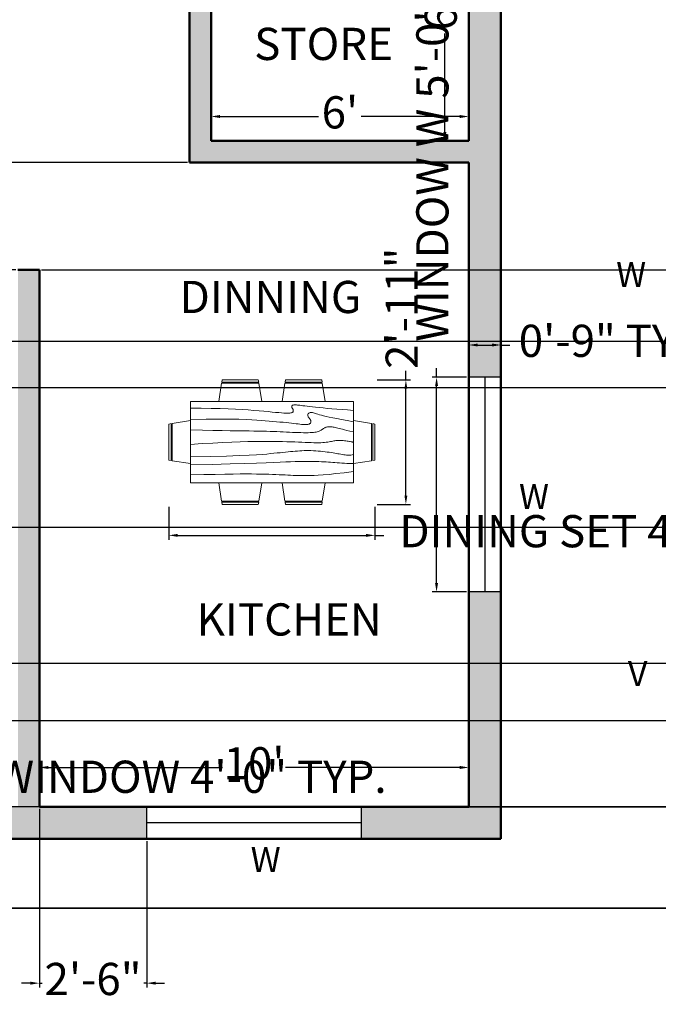
# Model space of a CAD drawing. Units: inches. Extents: x 2463 to 3327, y 6994 to 7582.
# Tile 2 of 5: x 2739 to 2917, y 6995 to 7270. Entities that reach past the tile are written whole.
import ezdxf

# ---------------------------------------------------------------- set-up
doc = ezdxf.new("R2010")
doc.units = ezdxf.units.IN
for name, color, linetype, lineweight in [('A-ANNO-DIMS', 2, 'Continuous', 18), ('A-ANNO-TEXT', 7, 'Continuous', 18), ('A-ANNO-TTLB', 7, 'Continuous', 35), ('A-AREA-IDEN', 3, 'Continuous', 25), ('A-FURN', 8, 'Continuous', 18), ('A-GLAZ', 4, 'Continuous', 25), ('A-WALL', 7, 'Continuous', 50), ('A-WALL-PATT', 252, 'Continuous', 13)]:
    doc.layers.add(name, color=color, linetype=linetype, lineweight=lineweight)
doc.styles.get("Standard").update_dxf_attribs({"font": 'times.ttf'})
doc.dimstyles.new('ISO-25', dxfattribs={"dimtxt": 9, "dimasz": 2.5, "dimexe": 1.25, "dimexo": 0.625, "dimgap": 2, "dimtad": 0, "dimdec": 1, "dimlunit": 4, "dimtxsty": 'Standard', "dimcen": 2.5, "dimadec": 0, "dimazin": 0, "dimtfac": 1, "dimtdec": 1, "dimtmove": 0, "dimatfit": 3, "dimfxl": 1, "dimarcsym": 0})

# ---------------------------------------------------------------- blocks, each defined once
blk = doc.blocks.new('*D3')
at = {"layer": 'A-ANNO-DIMS', "color": 0, "lineweight": -2, "transparency": 16777216}
for p, q in [((2863.81, 7307.83), (2856.5, 7307.83)), ((2857.75, 7305.33), (2857.75, 7277.78)), ((2857.75, 7238.33), (2857.75, 7265.87)), ((2863.81, 7235.83), (2856.5, 7235.83))]:
    blk.add_line(p, q, dxfattribs=at)
at = {"layer": 'A-ANNO-DIMS', "color": 0, "transparency": 16777216}
for points in [[(2857.34, 7305.33), (2858.17, 7305.33), (2857.75, 7307.83)], [(2857.34, 7238.33), (2858.17, 7238.33), (2857.75, 7235.83)]]:
    blk.add_solid(points, dxfattribs=at)
at = {"layer": 'Defpoints', "color": 0, "transparency": 16777216}
for p in [(2857.75, 7307.83), (2864.43, 7307.83), (2864.43, 7235.83)]:
    blk.add_point(p, dxfattribs=at)
at = {"layer": 'A-ANNO-DIMS', "color": 0, "transparency": 16777216, "insert": (2857.75, 7271.83), "char_height": 9, "attachment_point": 5, "rotation": 90}
blk.add_mtext("6'", dxfattribs=at)
blk = doc.blocks.new('*D4')
at = {"layer": 'A-ANNO-DIMS', "color": 0, "lineweight": -2, "transparency": 16777216}
for p, q in [((2792.43, 7236.45), (2792.43, 7243.92)), ((2864.43, 7236.45), (2864.43, 7243.92)), ((2794.93, 7242.67), (2822.48, 7242.67)), ((2861.93, 7242.67), (2834.38, 7242.67))]:
    blk.add_line(p, q, dxfattribs=at)
at = {"layer": 'A-ANNO-DIMS', "color": 0, "transparency": 16777216}
for points in [[(2794.93, 7243.09), (2794.93, 7242.25), (2792.43, 7242.67)], [(2861.93, 7243.09), (2861.93, 7242.25), (2864.43, 7242.67)]]:
    blk.add_solid(points, dxfattribs=at)
at = {"layer": 'Defpoints', "color": 0, "transparency": 16777216}
for p in [(2864.43, 7242.67), (2792.43, 7235.83), (2864.43, 7235.83)]:
    blk.add_point(p, dxfattribs=at)
at = {"layer": 'A-ANNO-DIMS', "color": 0, "transparency": 16777216, "insert": (2828.43, 7242.67), "char_height": 9, "attachment_point": 5}
blk.add_mtext("6'", dxfattribs=at)
blk = doc.blocks.new('*D5')
at = {"layer": 'A-ANNO-DIMS', "color": 0, "lineweight": -2, "transparency": 16777216}
for p, q in [((2744.43, 7050.45), (2744.43, 7062.04)), ((2864.43, 7050.45), (2864.43, 7062.04)), ((2746.93, 7060.79), (2795.65, 7060.79)), ((2861.93, 7060.79), (2813.21, 7060.79))]:
    blk.add_line(p, q, dxfattribs=at)
at = {"layer": 'A-ANNO-DIMS', "color": 0, "transparency": 16777216}
for points in [[(2746.93, 7061.21), (2746.93, 7060.38), (2744.43, 7060.79)], [(2861.93, 7061.21), (2861.93, 7060.38), (2864.43, 7060.79)]]:
    blk.add_solid(points, dxfattribs=at)
at = {"layer": 'Defpoints', "color": 0, "transparency": 16777216}
for p in [(2864.43, 7060.79), (2744.43, 7049.83), (2864.43, 7049.83)]:
    blk.add_point(p, dxfattribs=at)
at = {"layer": 'A-ANNO-DIMS', "color": 0, "transparency": 16777216, "insert": (2804.43, 7060.79), "char_height": 9, "attachment_point": 5}
blk.add_mtext("10'", dxfattribs=at)
blk = doc.blocks.new('Dining Set - 36 x 72 in.')
for p, q in [((-22, 27.5), (-22.1562, 26.50042)), ((-5.8416, 26.5), (-22.1534, 26.5)), ((-22, 27.5), (-6, 27.5)), ((-5.8437, 26.49966), (-6, 27.5)), ((6, 27.5), (5.8438, 26.50042)), ((22.1584, 26.5), (5.8466, 26.5)), ((6, 27.5), (22, 27.5)), ((22.1563, 26.49966), (22, 27.5)), ((-22.2343, 26.00059), (-23.4847, 17.99762)), ((-22.2304, 26), (-5.7608, 26)), ((-4.5152, 17.99762), (-5.7655, 25.99926)), ((5.7657, 26.00059), (4.5153, 17.99762)), ((5.7696, 26), (22.2392, 26)), ((23.4848, 17.99762), (22.2345, 25.99926)), ((36, 18), (-36, 18)), ((-36, 18), (-36, -18)), ((36, -18), (36, 18)), ((-44.0006, 8.23428), (-35.9976, 9.48474)), ((44.0006, 8.23428), (35.9976, 9.48474)), ((-45.5, 8), (-44.5004, 8.15617)), ((-45.5, 8), (-45.5, -8)), ((-44.5, -8.15843), (-44.5, 8.15338)), ((-44, 8.23041), (-44, -8.23915)), ((44, 8.23041), (44, -8.23915)), ((44.5, -8.15843), (44.5, 8.15338)), ((45.5, 8), (44.5005, 8.15617)), ((45.5, 8), (45.5, -8)), ((-44.4997, -8.15631), (-45.5, -8)), ((-35.9976, -9.48476), (-43.9993, -8.2345)), ((35.9976, -9.48476), (43.9993, -8.2345)), ((44.4997, -8.15631), (45.5, -8)), ((-36, -18), (36, -18)), ((-22.2343, -26.0006), (-23.4847, -17.99762)), ((-4.5152, -17.99762), (-5.7655, -25.99928)), ((5.7657, -26.0006), (4.5153, -17.99762)), ((23.4848, -17.99762), (22.2345, -25.99928)), ((-22.2304, -26), (-5.7608, -26)), ((5.7696, -26), (22.2392, -26)), ((-22, -27.5), (-22.1562, -26.50044)), ((-5.8416, -26.5), (-22.1534, -26.5)), ((-22, -27.5), (-6, -27.5)), ((-5.8437, -26.49967), (-6, -27.5)), ((6, -27.5), (5.8438, -26.50044)), ((22.1584, -26.5), (5.8466, -26.5)), ((6, -27.5), (22, -27.5)), ((22.1563, -26.49967), (22, -27.5))]:
    blk.add_line(p, q)
for points in [[(-36, 15), (-31.1772, 14.97754), (-26.8079, 14.91406), (-22.8538, 14.81543), (-19.276, 14.6875), (-16.0362, 14.53613), (-13.0957, 14.36718), (-10.4159, 14.18652), (-7.9583, 14), (-5.6904, 13.81315), (-3.6035, 13.63021), (-1.6954, 13.45508), (0.0365, 13.29166), (1.5945, 13.14388), (2.9811, 13.01562), (4.1988, 12.9108), (5.25, 12.83333), (6.1393, 12.78613), (6.8802, 12.76823), (7.4883, 12.77767), (7.9792, 12.8125), (8.3685, 12.87077), (8.6719, 12.95052), (8.9049, 13.0498), (9.0833, 13.16666), (9.2205, 13.29899), (9.3216, 13.44401), (9.3895, 13.59879), (9.4271, 13.76041), (9.4373, 13.92594), (9.4232, 14.09245), (9.3875, 14.257), (9.3333, 14.41666), (9.2638, 14.56917), (9.1836, 14.71484), (9.0975, 14.85465), (9.0104, 14.98958), (8.9272, 15.1206), (8.8529, 15.2487), (8.7922, 15.37483), (8.75, 15.5), (8.7305, 15.62467), (8.7344, 15.74739), (8.7617, 15.86621), (8.8125, 15.97916), (8.8867, 16.08431), (8.9844, 16.17968), (9.1055, 16.26334), (9.25, 16.33333), (9.4189, 16.38802), (9.6172, 16.42708), (9.8506, 16.45052), (10.125, 16.45833), (10.4463, 16.45052), (10.8203, 16.42708), (11.2529, 16.38802), (11.75, 16.33333), (12.3184, 16.26318), (12.9694, 16.17838), (13.7151, 16.07991), (14.5677, 15.96875), (15.5395, 15.84586), (16.6426, 15.71224), (17.8893, 15.56884), (19.2917, 15.41666), (20.859, 15.25667), (22.5879, 15.08984), (24.4721, 14.91715), (26.5052, 14.73958), (28.6809, 14.5581), (30.9929, 14.3737), (33.4347, 14.18733), (36, 14)], [(-36, 10), (-28.9766, 10.14274), (-23.1725, 10.20442), (-18.4241, 10.19775), (-14.5677, 10.13541), (-11.4399, 10.03011), (-8.877, 9.89453), (-6.7154, 9.74137), (-4.7917, 9.58333), (-2.9698, 9.43082), (-1.2246, 9.28515), (0.4415, 9.14534), (2.026, 9.01041), (3.5266, 8.87939), (4.9408, 8.7513), (6.266, 8.62516), (7.5, 8.5), (8.6411, 8.37549), (9.6914, 8.2539), (10.6538, 8.13818), (11.5312, 8.03125), (12.3267, 7.93603), (13.043, 7.85547), (13.6831, 7.79248), (14.25, 7.75), (14.7471, 7.7303), (15.1797, 7.73307), (15.5537, 7.75732), (15.875, 7.80208), (16.1494, 7.86637), (16.3828, 7.94922), (16.5811, 8.04964), (16.75, 8.16666), (16.8944, 8.29915), (17.0143, 8.44531), (17.1089, 8.60319), (17.1771, 8.77083), (17.218, 8.94629), (17.2305, 9.1276), (17.2137, 9.31282), (17.1667, 9.5), (17.0895, 9.6875), (16.987, 9.875), (16.8649, 10.0625), (16.7292, 10.25), (16.5856, 10.4375), (16.4401, 10.625), (16.2985, 10.8125), (16.1667, 11), (16.05, 11.18733), (15.9518, 11.3737), (15.8752, 11.5581), (15.8229, 11.73958), (15.798, 11.91715), (15.8034, 12.08984), (15.842, 12.25667), (15.9167, 12.41666), (16.0295, 12.56836), (16.1784, 12.70833), (16.3605, 12.83268), (16.5729, 12.9375), (16.8127, 13.01888), (17.0768, 13.07291), (17.3625, 13.0957), (17.6667, 13.08333), (17.9894, 13.03312), (18.3418, 12.94726), (18.7382, 12.82918), (19.1927, 12.68229), (19.7195, 12.51001), (20.3327, 12.31575), (21.0465, 12.10294), (21.875, 11.875), (22.8357, 11.63354), (23.959, 11.37304), (25.2786, 11.08618), (26.8282, 10.76562), (28.6414, 10.40405), (30.752, 9.99414), (33.1936, 9.52856), (36, 9)], [(-36, 5.5), (-30.7157, 5.3348), (-26.069, 5.20963), (-21.9946, 5.11767), (-18.4271, 5.05208), (-15.3009, 5.00602), (-12.5508, 4.97265), (-10.1112, 4.94515), (-7.9167, 4.91666), (-5.909, 4.88167), (-4.0586, 4.83984), (-2.3429, 4.79215), (-0.7396, 4.73958), (0.7739, 4.6831), (2.22, 4.6237), (3.6213, 4.56233), (5, 4.5), (6.373, 4.43782), (7.7344, 4.3776), (9.0723, 4.32129), (10.375, 4.27083), (11.6309, 4.22819), (12.8281, 4.19531), (13.9551, 4.17415), (15, 4.16666), (15.954, 4.17448), (16.819, 4.19791), (17.6001, 4.23698), (18.3021, 4.29166), (18.9299, 4.36198), (19.4883, 4.44791), (19.9823, 4.54948), (20.4167, 4.66666), (20.7969, 4.79899), (21.1302, 4.94401), (21.4245, 5.09879), (21.6875, 5.26041), (21.9271, 5.42594), (22.1511, 5.59245), (22.3672, 5.757), (22.5834, 5.91666), (22.8065, 6.06868), (23.0404, 6.21093), (23.2879, 6.34147), (23.5521, 6.45833), (23.8358, 6.55957), (24.142, 6.64323), (24.4735, 6.70735), (24.8334, 6.75), (25.2235, 6.76969), (25.642, 6.76692), (26.0858, 6.74267), (26.5521, 6.69791), (27.0379, 6.63362), (27.5404, 6.55078), (28.0565, 6.45036), (28.5834, 6.33333), (29.1242, 6.19987), (29.7071, 6.04687), (30.3661, 5.87044), (31.1354, 5.66666), (32.0493, 5.43164), (33.142, 5.16146), (34.4475, 4.85221), (36, 4.5)], [(-36, -1), (-30.7915, -0.6591), (-26.0195, -0.38216), (-21.6519, -0.16284), (-17.6563, 0.00521), (-14.0005, 0.12833), (-10.6523, 0.21289), (-7.5796, 0.26522), (-4.75, 0.29166), (-2.134, 0.29793), (0.2878, 0.28711), (2.5317, 0.26163), (4.6146, 0.22396), (6.5529, 0.17651), (8.3633, 0.12174), (10.0623, 0.06209), (11.6667, 0), (13.1899, -0.06201), (14.6341, -0.1211), (15.9982, -0.17432), (17.2813, -0.21875), (18.4823, -0.25147), (19.6003, -0.26953), (20.6343, -0.27002), (21.5834, -0.25), (22.4481, -0.20768), (23.2357, -0.14584), (23.9549, -0.06836), (24.6146, 0.02083), (25.2235, 0.11784), (25.7904, 0.21875), (26.3241, 0.31966), (26.8334, 0.41666), (27.3265, 0.50618), (27.8099, 0.58593), (28.2894, 0.65397), (28.7709, 0.70833), (29.2601, 0.74707), (29.763, 0.76823), (30.2855, 0.76985), (30.8334, 0.75), (31.4088, 0.70784), (31.9994, 0.64713), (32.589, 0.57275), (33.1615, 0.48958), (33.7008, 0.4025), (34.1908, 0.3164), (34.6153, 0.23616), (34.9584, 0.16666), (35.2099, 0.11165), (35.3848, 0.07031), (35.504, 0.04069), (35.5886, 0.02083), (35.6594, 0.00879), (35.7377, 0.0026), (35.8442, 0.00032), (36, 0)], [(-36, -6.5), (-27.1843, -6.31267), (-20.084, -6.1263), (-14.469, -5.9419), (-10.1094, -5.76042), (-6.7752, -5.58285), (-4.2363, -5.41016), (-2.2629, -5.24333), (-0.625, -5.08334), (0.8708, -4.93099), (2.2715, -4.78646), (3.5872, -4.64974), (4.8281, -4.52084), (6.0046, -4.39974), (7.127, -4.28646), (8.2053, -4.18099), (9.25, -4.08334), (10.2705, -3.99382), (11.2734, -3.91407), (12.2647, -3.84603), (13.25, -3.79167), (14.2354, -3.75293), (15.2266, -3.73177), (16.2295, -3.73015), (17.25, -3.75), (18.2912, -3.79248), (19.3451, -3.85547), (20.4009, -3.93604), (21.4479, -4.03125), (22.4754, -4.13819), (23.4727, -4.25391), (24.4289, -4.37549), (25.3334, -4.5), (26.1785, -4.62492), (26.9694, -4.74935), (27.7145, -4.87281), (28.4219, -4.99479), (29.1, -5.11483), (29.7572, -5.23242), (30.4016, -5.34709), (31.0417, -5.45834), (31.6837, -5.56437), (32.3262, -5.65821), (32.9658, -5.73153), (33.599, -5.77604), (34.2224, -5.78345), (34.8327, -5.74545), (35.4264, -5.65373), (36, -5.5)], [(-36, -10), (-26.4022, -9.81299), (-18.4675, -9.62891), (-11.9839, -9.45069), (-6.7396, -9.28125), (-2.5226, -9.12354), (0.8789, -8.98047), (3.6769, -8.85498), (6.0833, -8.75), (8.2767, -8.66765), (10.3021, -8.60677), (12.1712, -8.56543), (13.8958, -8.54167), (15.4876, -8.53353), (16.9583, -8.53907), (18.3197, -8.55632), (19.5834, -8.58334), (20.7616, -8.61841), (21.8685, -8.66081), (22.9188, -8.71004), (23.9271, -8.76563), (24.9081, -8.82707), (25.8763, -8.89388), (26.8465, -8.96558), (27.8334, -9.04167), (28.8474, -9.12118), (29.8828, -9.20117), (30.93, -9.27824), (31.9792, -9.34896), (33.0205, -9.40991), (34.0443, -9.45768), (35.0407, -9.48885), (36, -9.5)], [(-36, -14.5), (-30.0881, -14.33513), (-25.0332, -14.21224), (-20.7312, -14.12647), (-17.0781, -14.07292), (-13.97, -14.04671), (-11.3027, -14.04297), (-8.9724, -14.05681), (-6.875, -14.08334), (-4.9224, -14.11833), (-3.0905, -14.16016), (-1.3709, -14.20785), (0.2448, -14.26042), (1.7647, -14.3169), (3.1973, -14.3763), (4.5507, -14.43767), (5.8333, -14.5), (7.0554, -14.5621), (8.235, -14.62175), (9.3922, -14.67652), (10.5469, -14.72396), (11.7192, -14.76164), (12.929, -14.78711), (14.1965, -14.79794), (15.5417, -14.79167), (16.9933, -14.76424), (18.6152, -14.70508), (20.4804, -14.60197), (22.6615, -14.44271), (25.2312, -14.21509), (28.2624, -13.9069), (31.8277, -13.50594), (36, -13)]]:
    blk.add_lwpolyline(points)
blk = doc.blocks.new('WIN-60')
for p, q in [((9, 60), (0, 60)), ((4.5, 60), (4.5, 0)), ((9, 0), (0, 0))]:
    blk.add_line(p, q)
blk = doc.blocks.new('*D35')
at = {"layer": 'A-ANNO-DIMS', "color": 0, "lineweight": -2, "transparency": 16777216}
for p, q in [((2780.62, 7133.65), (2780.62, 7124.39)), ((2838.22, 7133.65), (2838.22, 7124.39)), ((2783.12, 7125.64), (2835.72, 7125.64)), ((2838.22, 7125.64), (2840.72, 7125.64))]:
    blk.add_line(p, q, dxfattribs=at)
at = {"layer": 'A-ANNO-DIMS', "color": 0, "transparency": 16777216}
for points in [[(2783.12, 7126.06), (2783.12, 7125.22), (2780.62, 7125.64)], [(2835.72, 7126.06), (2835.72, 7125.22), (2838.22, 7125.64)]]:
    blk.add_solid(points, dxfattribs=at)
at = {"layer": 'Defpoints', "color": 0, "transparency": 16777216}
for p in [(2780.62, 7134.28), (2838.22, 7134.28), (2838.22, 7125.64)]:
    blk.add_point(p, dxfattribs=at)
at = {"layer": 'A-ANNO-DIMS', "color": 0, "transparency": 16777216, "insert": (2903.83, 7125.64), "char_height": 9, "attachment_point": 5}
blk.add_mtext('DINING SET 4\'-9 1/2"', dxfattribs=at)
blk = doc.blocks.new('*D36')
at = {"layer": 'A-ANNO-DIMS', "color": 0, "lineweight": -2, "transparency": 16777216}
for p, q in [((2846.86, 7169.09), (2846.86, 7171.59)), ((2838.84, 7169.09), (2848.11, 7169.09)), ((2846.86, 7136.78), (2846.86, 7166.59)), ((2838.84, 7134.28), (2848.11, 7134.28))]:
    blk.add_line(p, q, dxfattribs=at)
at = {"layer": 'A-ANNO-DIMS', "color": 0, "transparency": 16777216}
for points in [[(2846.44, 7166.59), (2847.27, 7166.59), (2846.86, 7169.09)], [(2846.44, 7136.78), (2847.27, 7136.78), (2846.86, 7134.28)]]:
    blk.add_solid(points, dxfattribs=at)
at = {"layer": 'Defpoints', "color": 0, "transparency": 16777216}
for p in [(2838.22, 7169.09), (2846.86, 7169.09), (2838.22, 7134.28)]:
    blk.add_point(p, dxfattribs=at)
at = {"layer": 'A-ANNO-DIMS', "color": 0, "transparency": 16777216, "insert": (2846.86, 7189.1), "char_height": 9, "attachment_point": 5, "rotation": 90}
blk.add_mtext('2\'-11"', dxfattribs=at)
blk = doc.blocks.new('*D37')
at = {"layer": 'A-ANNO-DIMS', "color": 0, "lineweight": -2, "transparency": 16777216}
for p, q in [((2855.43, 7169.83), (2855.43, 7172.33)), ((2863.81, 7169.83), (2854.18, 7169.83)), ((2855.43, 7112.33), (2855.43, 7167.33)), ((2863.81, 7109.83), (2854.18, 7109.83))]:
    blk.add_line(p, q, dxfattribs=at)
at = {"layer": 'A-ANNO-DIMS', "color": 0, "transparency": 16777216}
for points in [[(2855.01, 7167.33), (2855.85, 7167.33), (2855.43, 7169.83)], [(2855.01, 7112.33), (2855.85, 7112.33), (2855.43, 7109.83)]]:
    blk.add_solid(points, dxfattribs=at)
at = {"layer": 'Defpoints', "color": 0, "transparency": 16777216}
for p in [(2855.43, 7169.83), (2864.43, 7169.83), (2864.43, 7109.83)]:
    blk.add_point(p, dxfattribs=at)
at = {"layer": 'A-ANNO-DIMS', "color": 0, "transparency": 16777216, "insert": (2855.43, 7241.15), "char_height": 9, "attachment_point": 5, "rotation": 90}
blk.add_mtext('WINDOW W 5\'-0" TYP.', dxfattribs=at)
blk = doc.blocks.new('*D38')
at = {"layer": 'A-ANNO-DIMS', "color": 0, "lineweight": -2, "transparency": 16777216}
for p, q in [((2864.43, 7170.45), (2864.43, 7180.08)), ((2866.93, 7178.83), (2870.93, 7178.83)), ((2873.43, 7170.45), (2873.43, 7180.08)), ((2873.43, 7178.83), (2875.93, 7178.83))]:
    blk.add_line(p, q, dxfattribs=at)
at = {"layer": 'A-ANNO-DIMS', "color": 0, "transparency": 16777216}
for points in [[(2866.93, 7179.24), (2866.93, 7178.41), (2864.43, 7178.83)], [(2870.93, 7179.24), (2870.93, 7178.41), (2873.43, 7178.83)]]:
    blk.add_solid(points, dxfattribs=at)
at = {"layer": 'Defpoints', "color": 0, "transparency": 16777216}
for p in [(2873.43, 7178.83), (2864.43, 7169.83), (2873.43, 7169.83)]:
    blk.add_point(p, dxfattribs=at)
at = {"layer": 'A-ANNO-DIMS', "color": 0, "transparency": 16777216, "insert": (2905.86, 7178.83), "char_height": 9, "attachment_point": 5}
blk.add_mtext('0\'-9" TYP.', dxfattribs=at)
blk = doc.blocks.new('*D41')
at = {"layer": 'A-ANNO-DIMS', "color": 0, "lineweight": -2, "transparency": 16777216}
for p, q in [((2675.43, 7050.45), (2675.43, 7058.28)), ((2677.93, 7057.03), (2720.93, 7057.03)), ((2723.43, 7050.45), (2723.43, 7058.28)), ((2723.43, 7057.03), (2725.93, 7057.03))]:
    blk.add_line(p, q, dxfattribs=at)
at = {"layer": 'A-ANNO-DIMS', "color": 0, "transparency": 16777216}
for points in [[(2677.93, 7057.44), (2677.93, 7056.61), (2675.43, 7057.03)], [(2720.93, 7057.44), (2720.93, 7056.61), (2723.43, 7057.03)]]:
    blk.add_solid(points, dxfattribs=at)
at = {"layer": 'Defpoints', "color": 0, "transparency": 16777216}
for p in [(2723.43, 7057.03), (2675.43, 7049.83), (2723.43, 7049.83)]:
    blk.add_point(p, dxfattribs=at)
at = {"layer": 'A-ANNO-DIMS', "color": 0, "transparency": 16777216, "insert": (2786.83, 7057.03), "char_height": 9, "attachment_point": 5}
blk.add_mtext('WINDOW 4\'-0" TYP.', dxfattribs=at)
blk = doc.blocks.new('*D52')
at = {"layer": 'A-ANNO-DIMS', "color": 0, "lineweight": -2, "transparency": 16777216}
for p, q in [((2660.43, 7272.45), (2660.43, 7562.38)), ((2662.93, 7561.13), (2706.56, 7561.13)), ((2783.93, 7561.13), (2740.3, 7561.13)), ((2786.43, 7230.45), (2786.43, 7562.38))]:
    blk.add_line(p, q, dxfattribs=at)
at = {"layer": 'A-ANNO-DIMS', "color": 0, "transparency": 16777216}
for points in [[(2662.93, 7561.54), (2662.93, 7560.71), (2660.43, 7561.13)], [(2783.93, 7561.54), (2783.93, 7560.71), (2786.43, 7561.13)]]:
    blk.add_solid(points, dxfattribs=at)
at = {"layer": 'Defpoints', "color": 0, "transparency": 16777216}
for p in [(2786.43, 7561.13), (2660.43, 7271.83), (2786.43, 7229.83)]:
    blk.add_point(p, dxfattribs=at)
at = {"layer": 'A-ANNO-DIMS', "color": 0, "transparency": 16777216, "insert": (2723.43, 7561.13), "char_height": 9, "attachment_point": 5}
blk.add_mtext('10\'-6"', dxfattribs=at)
blk = doc.blocks.new('*D53')
at = {"layer": 'A-ANNO-DIMS', "color": 0, "lineweight": -2, "transparency": 16777216}
for p, q in [((2473.13, 7232.33), (2473.13, 7234.83)), ((2785.81, 7229.83), (2471.88, 7229.83)), ((2473.13, 7229.83), (2473.13, 7229.01)), ((2737.81, 7199.83), (2471.88, 7199.83)), ((2473.13, 7199.83), (2473.13, 7200.64)), ((2473.13, 7197.33), (2473.13, 7194.83))]:
    blk.add_line(p, q, dxfattribs=at)
at = {"layer": 'A-ANNO-DIMS', "color": 0, "transparency": 16777216}
for points in [[(2472.71, 7232.33), (2473.55, 7232.33), (2473.13, 7229.83)], [(2472.71, 7197.33), (2473.55, 7197.33), (2473.13, 7199.83)]]:
    blk.add_solid(points, dxfattribs=at)
at = {"layer": 'Defpoints', "color": 0, "transparency": 16777216}
for p in [(2473.13, 7229.83), (2786.43, 7229.83), (2738.43, 7199.83)]:
    blk.add_point(p, dxfattribs=at)
at = {"layer": 'A-ANNO-DIMS', "color": 0, "transparency": 16777216, "insert": (2473.13, 7214.83), "char_height": 9, "attachment_point": 5, "rotation": 90}
blk.add_mtext('2\'-6"', dxfattribs=at)
blk = doc.blocks.new('*D59')
at = {"layer": 'A-ANNO-DIMS', "color": 0, "lineweight": -2, "transparency": 16777216}
for p, q in [((2745.06, 7199.83), (3321.97, 7199.83)), ((3320.72, 7197.33), (3320.72, 7141.69)), ((3320.72, 7052.33), (3320.72, 7107.96)), ((2745.06, 7049.83), (3321.97, 7049.83))]:
    blk.add_line(p, q, dxfattribs=at)
at = {"layer": 'A-ANNO-DIMS', "color": 0, "transparency": 16777216}
for points in [[(3320.31, 7197.33), (3321.14, 7197.33), (3320.72, 7199.83)], [(3320.31, 7052.33), (3321.14, 7052.33), (3320.72, 7049.83)]]:
    blk.add_solid(points, dxfattribs=at)
at = {"layer": 'Defpoints', "color": 0, "transparency": 16777216}
for p in [(2744.43, 7199.83), (2744.43, 7049.83), (3320.72, 7049.83)]:
    blk.add_point(p, dxfattribs=at)
at = {"layer": 'A-ANNO-DIMS', "color": 0, "transparency": 16777216, "insert": (3320.72, 7124.83), "char_height": 9, "attachment_point": 5, "rotation": 90}
blk.add_mtext('12\'-6"', dxfattribs=at)
blk = doc.blocks.new('*D67')
at = {"layer": 'A-ANNO-DIMS', "color": 0, "lineweight": -2, "transparency": 16777216}
for p, q in [((2744.43, 7049.2), (2744.43, 6999.28)), ((2774.43, 7040.2), (2774.43, 6999.28)), ((2741.93, 7000.53), (2739.43, 7000.53)), ((2744.43, 7000.53), (2745.25, 7000.53)), ((2774.43, 7000.53), (2773.61, 7000.53)), ((2776.93, 7000.53), (2779.43, 7000.53))]:
    blk.add_line(p, q, dxfattribs=at)
at = {"layer": 'A-ANNO-DIMS', "color": 0, "transparency": 16777216}
for points in [[(2741.93, 7000.94), (2741.93, 7000.11), (2744.43, 7000.53)], [(2776.93, 7000.94), (2776.93, 7000.11), (2774.43, 7000.53)]]:
    blk.add_solid(points, dxfattribs=at)
at = {"layer": 'Defpoints', "color": 0, "transparency": 16777216}
for p in [(2744.43, 7049.83), (2774.43, 7040.83), (2774.43, 7000.53)]:
    blk.add_point(p, dxfattribs=at)
at = {"layer": 'A-ANNO-DIMS', "color": 0, "transparency": 16777216, "insert": (2759.43, 7000.53), "char_height": 9, "attachment_point": 5}
blk.add_mtext('2\'-6"', dxfattribs=at)
blk = doc.blocks.new('*D75')
at = {"layer": 'A-ANNO-DIMS', "color": 0, "lineweight": -2, "transparency": 16777216}
for p, q in [((3144.8, 7179.83), (2471.88, 7179.83)), ((2473.13, 7177.33), (2473.13, 7148.9)), ((2473.13, 7092.33), (2473.13, 7120.75)), ((3144.8, 7089.83), (2471.88, 7089.83))]:
    blk.add_line(p, q, dxfattribs=at)
at = {"layer": 'A-ANNO-DIMS', "color": 0, "transparency": 16777216}
for points in [[(2472.71, 7177.33), (2473.55, 7177.33), (2473.13, 7179.83)], [(2472.71, 7092.33), (2473.55, 7092.33), (2473.13, 7089.83)]]:
    blk.add_solid(points, dxfattribs=at)
at = {"layer": 'Defpoints', "color": 0, "transparency": 16777216}
for p in [(3145.42, 7179.83), (2473.13, 7089.83), (3145.42, 7089.83)]:
    blk.add_point(p, dxfattribs=at)
at = {"layer": 'A-ANNO-DIMS', "color": 0, "transparency": 16777216, "insert": (2473.13, 7134.83), "char_height": 9, "attachment_point": 5, "rotation": 90}
blk.add_mtext('7\'-6"', dxfattribs=at)
blk = doc.blocks.new('*D76')
at = {"layer": 'A-ANNO-DIMS', "color": 0, "lineweight": -2, "transparency": 16777216}
for p, q in [((2473.13, 7073.83), (2473.13, 7076.33)), ((2928.8, 7073.83), (2471.88, 7073.83)), ((2473.13, 7052.33), (2473.13, 7071.33)), ((2928.8, 7049.83), (2471.88, 7049.83))]:
    blk.add_line(p, q, dxfattribs=at)
at = {"layer": 'A-ANNO-DIMS', "color": 0, "transparency": 16777216}
for points in [[(2472.71, 7071.33), (2473.55, 7071.33), (2473.13, 7073.83)], [(2472.71, 7052.33), (2473.55, 7052.33), (2473.13, 7049.83)]]:
    blk.add_solid(points, dxfattribs=at)
at = {"layer": 'Defpoints', "color": 0, "transparency": 16777216}
for p in [(2473.13, 7073.83), (2929.42, 7073.83), (2929.42, 7049.83)]:
    blk.add_point(p, dxfattribs=at)
at = {"layer": 'A-ANNO-DIMS', "color": 0, "transparency": 16777216, "insert": (2473.13, 7090.51), "char_height": 9, "attachment_point": 5, "rotation": 90}
blk.add_mtext('2\'-0"', dxfattribs=at)
blk = doc.blocks.new('*D77')
at = {"layer": 'A-ANNO-DIMS', "color": 0, "lineweight": -2, "transparency": 16777216}
for p, q in [((2928.8, 7166.83), (2471.88, 7166.83)), ((2473.13, 7164.33), (2473.13, 7161.38)), ((2473.13, 7130.33), (2473.13, 7133.27)), ((2928.8, 7127.83), (2471.88, 7127.83))]:
    blk.add_line(p, q, dxfattribs=at)
at = {"layer": 'A-ANNO-DIMS', "color": 0, "transparency": 16777216}
for points in [[(2472.71, 7164.33), (2473.55, 7164.33), (2473.13, 7166.83)], [(2472.71, 7130.33), (2473.55, 7130.33), (2473.13, 7127.83)]]:
    blk.add_solid(points, dxfattribs=at)
at = {"layer": 'Defpoints', "color": 0, "transparency": 16777216}
for p in [(2473.13, 7166.83), (2929.42, 7166.83), (2929.42, 7127.83)]:
    blk.add_point(p, dxfattribs=at)
at = {"layer": 'A-ANNO-DIMS', "color": 0, "transparency": 16777216, "insert": (2473.13, 7147.33), "char_height": 9, "attachment_point": 5, "rotation": 90}
blk.add_mtext('3\'-3"', dxfattribs=at)

msp = doc.modelspace()

# ---------------------------------------------------------------- hatches: boundary and pattern name
at = {"layer": 'A-WALL-PATT'}
h = msp.add_hatch(color=256, dxfattribs=at)
h.dxf.hatch_style = 1
h.paths.add_polyline_path([(2522.43, 7511.83), (2690.43, 7511.83), (2690.43, 7385.83), (2696.43, 7385.83), (2702.68, 7385.83), (2702.68, 7391.83), (2696.43, 7391.83), (2696.43, 7511.83), (2864.43, 7511.83), (2864.43, 7481.83), (2873.43, 7481.83), (2873.43, 7520.83), (2513.43, 7520.83), (2513.43, 7501.71), (2522.43, 7501.71)])
h.paths.add_polyline_path([(2522.43, 7453.71, -0.042779), (2513.43, 7453.71), (2513.43, 7392.77), (2522.43, 7392.77)], flags=0)
h.paths.add_polyline_path([(2522.43, 7332.77), (2513.43, 7332.77), (2513.43, 7226.83), (2522.43, 7226.83), (2522.43, 7265.83), (2654.43, 7265.83), (2654.43, 7263.42), (2660.43, 7263.42), (2660.43, 7271.83), (2522.43, 7271.83)])
h.paths.add_polyline_path([(2873.43, 7421.83), (2864.43, 7421.83), (2864.43, 7391.83), (2861.59, 7391.83), (2861.59, 7385.83), (2864.43, 7385.83), (2864.43, 7361.83), (2873.43, 7361.83)])
h.paths.add_polyline_path([(2792.43, 7385.83), (2831.59, 7385.83, -0.045361), (2831.59, 7391.83), (2738.68, 7391.83, -0.038405), (2738.68, 7385.83), (2786.43, 7385.83), (2786.43, 7313.83), (2786.43, 7307.83), (2786.43, 7305.07), (2792.43, 7305.07), (2792.43, 7307.83), (2864.43, 7307.83), (2864.43, 7235.83), (2792.43, 7235.83), (2792.43, 7275.07, -0.045361), (2786.43, 7275.07), (2786.43, 7235.83), (2786.43, 7229.83), (2864.43, 7229.83), (2864.43, 7169.83), (2873.43, 7169.83), (2873.43, 7337.83), (2864.43, 7337.83), (2864.43, 7313.83), (2792.43, 7313.83)])
h.paths.add_polyline_path([(2873.43, 7109.83), (2864.43, 7109.83), (2864.43, 7049.83), (2834.43, 7049.83), (2834.43, 7040.83), (2873.43, 7040.83)])
h.paths.add_polyline_path([(2774.43, 7049.83), (2744.43, 7049.83), (2744.43, 7199.83), (2738.43, 7199.83), (2738.43, 7049.83), (2723.43, 7049.83), (2723.43, 7040.83), (2774.43, 7040.83)])
h.paths.add_polyline_path([(2675.43, 7049.83), (2660.43, 7049.83), (2660.43, 7121.83), (2660.43, 7127.83), (2660.43, 7227.42, -0.038405), (2654.43, 7227.42), (2654.43, 7127.83), (2651.08, 7127.83), (2651.08, 7121.83), (2654.43, 7121.83), (2654.43, 7049.83), (2522.43, 7049.83), (2522.43, 7073.83), (2513.43, 7073.83), (2513.43, 7040.83), (2675.43, 7040.83)])
h.paths.add_polyline_path([(2621.08, 7127.83), (2522.43, 7127.83), (2522.43, 7166.83), (2513.43, 7166.83), (2513.43, 7097.83), (2522.43, 7097.83), (2522.43, 7121.83), (2621.08, 7121.83, -0.045361)], flags=17)
h.paths.add_polyline_path([(3280.42, 7520.83), (2920.42, 7520.83), (2920.42, 7501.71), (2929.42, 7501.71), (2929.42, 7511.83), (3097.42, 7511.83), (3097.42, 7385.83), (3103.42, 7385.83), (3109.67, 7385.83), (3109.67, 7391.83), (3103.42, 7391.83), (3103.42, 7511.83), (3271.42, 7511.83), (3271.42, 7481.83), (3280.42, 7481.83)])
h.paths.add_polyline_path([(3280.42, 7421.83), (3271.42, 7421.83), (3271.42, 7391.83), (3268.58, 7391.83), (3268.58, 7385.83), (3271.42, 7385.83), (3271.42, 7361.83), (3280.42, 7361.83)])
h.paths.add_polyline_path([(3238.58, 7391.83), (3145.67, 7391.83, -0.038405), (3145.67, 7385.83), (3193.42, 7385.83), (3193.42, 7313.83), (3193.42, 7307.83), (3193.42, 7305.07), (3199.42, 7305.07), (3199.42, 7307.83), (3271.42, 7307.83), (3271.42, 7235.83), (3199.42, 7235.83), (3193.42, 7235.83), (3193.42, 7229.83), (3271.42, 7229.83), (3280.42, 7229.83), (3280.42, 7337.83), (3271.42, 7337.83), (3271.42, 7313.83), (3199.42, 7313.83), (3199.42, 7385.83), (3238.58, 7385.83, -0.045361)])
h.paths.add_polyline_path([(3199.42, 7275.07, -0.045361), (3193.42, 7275.07), (3193.42, 7235.83), (3199.42, 7235.83)], flags=17)
h.paths.add_polyline_path([(3193.42, 7235.83), (3145.42, 7235.83), (3145.42, 7227.44), (3151.42, 7227.44), (3151.42, 7229.83), (3193.42, 7229.83)])
h.paths.add_polyline_path([(3151.42, 7199.83, -0.044871), (3145.42, 7199.83), (3145.42, 7049.83), (3130.42, 7049.83), (3130.42, 7040.83), (3151.42, 7040.83), (3151.42, 7049.83)])
h.paths.add_polyline_path([(3082.42, 7049.83), (3067.42, 7049.83), (3067.42, 7121.83), (3067.42, 7127.83), (3067.42, 7227.42, -0.038405), (3061.42, 7227.42), (3061.42, 7127.83), (3058.07, 7127.83), (3058.07, 7121.83), (3061.42, 7121.83), (3061.42, 7049.83), (2929.42, 7049.83), (2929.42, 7073.83), (2920.42, 7073.83), (2920.42, 7040.83), (3082.42, 7040.83)])
h.paths.add_polyline_path([(3028.07, 7121.83), (2997.56, 7121.83), (2997.56, 7113.83), (2991.06, 7113.83), (2993.06, 7107.83, -0.501323), (2988.1, 7088.96, -0.132891), (2986.01, 7088.96, -0.501317), (2981.06, 7107.83), (2983.06, 7113.83), (2980.06, 7113.83), (2980.06, 7112.33), (2977.06, 7112.33), (2977.06, 7113.83), (2976.56, 7113.83), (2976.56, 7121.83), (2929.42, 7121.83), (2929.42, 7097.83), (2920.42, 7097.83), (2920.42, 7166.83), (2929.42, 7166.83), (2929.42, 7127.83), (3028.07, 7127.83, 0.045361)], flags=17)
h.paths.add_polyline_path([(2995.56, 7120.83, -0.414214), (2996.56, 7120.08), (2996.56, 7115.83, -0.414214), (2995.81, 7114.83), (2978.56, 7114.83, -0.414214), (2977.56, 7115.58), (2977.56, 7119.83, -0.414214), (2978.31, 7120.83)], flags=16)
h.paths.add_polyline_path([(2988.7, 7090.3, -0.215004), (2985.41, 7090.3, -0.48008), (2983.06, 7107.83), (2991.06, 7107.83, -0.48008)], flags=16)
h.paths.add_polyline_path([(2929.42, 7265.83), (3061.42, 7265.83), (3061.42, 7263.42), (3067.42, 7263.42), (3067.42, 7271.83), (2929.42, 7271.83), (2929.42, 7332.77), (2920.42, 7332.77), (2920.42, 7226.83), (2929.42, 7226.83)])
h.paths.add_polyline_path([(2929.42, 7453.71, -0.042779), (2920.42, 7453.71), (2920.42, 7392.77), (2929.42, 7392.77)], flags=0)

# ---------------------------------------------------------------- linework, layer by layer
at = {"layer": 'A-ANNO-TTLB'}
msp.add_lwpolyline([(2463.47, 7549.29), (3297.67, 7549.29), (3297.67, 7021.48), (2463.47, 7021.48)], close=True, dxfattribs=at)
at = {"layer": 'A-WALL'}
for p, q in [((2873.43, 7520.83), (2873.43, 7040.83)), ((2786.43, 7307.83), (2786.43, 7235.83)), ((2864.43, 7307.83), (2864.43, 7235.83)), ((2792.43, 7275.07), (2792.43, 7235.83)), ((2786.43, 7235.83), (2786.43, 7229.83)), ((2792.43, 7235.83), (2864.43, 7235.83)), ((2786.43, 7229.83), (2864.43, 7229.83)), ((2864.43, 7229.83), (2864.43, 7049.83)), ((2738.43, 7199.83), (2744.43, 7199.83)), ((2744.43, 7199.83), (2744.43, 7049.83)), ((2864.43, 7049.83), (2744.43, 7049.83)), ((2873.43, 7040.83), (2513.43, 7040.83))]:
    msp.add_line(p, q, dxfattribs=at)

# ---------------------------------------------------------------- block references
at = {"layer": 'A-FURN', "xscale": 0.6329712530369104, "yscale": 0.6329712530369104, "zscale": 0.6329712530369104}
msp.add_blockref('Dining Set - 36 x 72 in.', (2809.42, 7151.69), dxfattribs=at)
at = {"layer": 'A-GLAZ'}
msp.add_blockref('WIN-60', (2864.43, 7109.83), dxfattribs=at)
at = {"layer": 'A-GLAZ', "rotation": 269.9999999999949}
msp.add_blockref('WIN-60', (2774.43, 7049.83), dxfattribs=at)

# ---------------------------------------------------------------- texts
at = {"layer": 'A-ANNO-TEXT', "char_height": 7, "attachment_point": 1}
for s, insert in [('\\pxqc;{\\fTimes New Roman|b1|i0|c0|p18;W}', (2895.62, 7202.06)), ('\\pxqc;{\\fTimes New Roman|b1|i0|c0|p18;W}', (2868.46, 7140)), ('\\pxqc;{\\fTimes New Roman|b1|i0|c0|p18;V}', (2897.44, 7090.55)), ('\\pxqc;{\\fTimes New Roman|b1|i0|c0|p18;W}', (2793.48, 7038.56))]:
    msp.add_mtext_dynamic_manual_height_columns(s, width=28.3852, gutter_width=12.5, heights=[0], dxfattribs=dict(at, insert=insert))
at = {"layer": 'A-AREA-IDEN', "char_height": 9, "attachment_point": 1}
for s, width, insert in [('\\pxqc;{\\fTimes New Roman|b1|i0|c0|p18;STORE}', 56.3539, (2795.69, 7267.46)), ('\\pxqc;{\\fTimes New Roman|b1|i0|c0|p18;DINNING}', 68.4707, (2774.76, 7196.75)), ('\\pxqc;{\\fTimes New Roman|b1|i0|c0|p18;KITCHEN}', 83.8599, (2772.31, 7106.65))]:
    msp.add_mtext_dynamic_manual_height_columns(s, width=width, gutter_width=12.5, heights=[0], dxfattribs=dict(at, insert=insert))

# ---------------------------------------------------------------- dimensions: what is measured, and where the dimension line sits
at = {"layer": 'A-ANNO-DIMS'}
for base, p1, p2, override, picture, middle in [((2786.43, 7561.13), (2660.43, 7271.83), (2786.43, 7229.83), {"dimdec": 1, "dimlfac": 1, "dimrnd": 0, "dimzin": 1, "dimdsep": 46, "dimlunit": 4, "dimfrac": 2}, '*D52', (2723.43, 7561.13)), ((2864.43, 7242.67), (2792.43, 7235.83), (2864.43, 7235.83), {"dimclrd": 0, "dimclre": 0, "dimclrt": 0}, '*D4', (2828.43, 7242.67)), ((2864.43, 7060.79), (2744.43, 7049.83), (2864.43, 7049.83), {"dimclrd": 0, "dimclre": 0, "dimclrt": 0}, '*D5', (2804.43, 7060.79)), ((2774.43, 7000.53), (2744.43, 7049.83), (2774.43, 7040.83), {"dimdec": 1, "dimlfac": 1, "dimrnd": 0, "dimzin": 1, "dimdsep": 46, "dimlunit": 4, "dimfrac": 2}, '*D67', (2759.43, 7000.53))]:
    dim = msp.add_linear_dim(base=base, p1=p1, p2=p2, dimstyle='ISO-25', override=override, dxfattribs=at)
    dim.commit()
    dim.dimension.update_dxf_attribs({"geometry": picture, "text_midpoint": middle})
for base, p1, p2, override, picture, middle in [((2857.75, 7307.83), (2864.43, 7235.83), (2864.43, 7307.83), {"dimclrd": 0, "dimclre": 0, "dimclrt": 0}, '*D3', (2857.75, 7271.83)), ((2473.13, 7229.83), (2738.43, 7199.83), (2786.43, 7229.83), {"dimdec": 1, "dimlfac": 1, "dimrnd": 0, "dimzin": 1, "dimdsep": 46, "dimlunit": 4, "dimfrac": 2}, '*D53', (2473.13, 7214.83)), ((2846.86, 7169.09), (2838.22, 7134.28), (2838.22, 7169.09), {"dimdec": 1, "dimrnd": 0, "dimzin": 1, "dimlunit": 4, "dimfrac": 2}, '*D36', (2846.86, 7189.1)), ((3320.72, 7049.83), (2744.43, 7199.83), (2744.43, 7049.83), {"dimdec": 1, "dimlfac": 1, "dimrnd": 0, "dimzin": 1, "dimdsep": 46, "dimlunit": 4, "dimfrac": 2}, '*D59', (3320.72, 7124.83)), ((2473.13, 7089.83), (3145.42, 7179.83), (3145.42, 7089.83), {"dimdec": 1, "dimlfac": 1, "dimrnd": 0, "dimzin": 1, "dimdsep": 46, "dimlunit": 4, "dimfrac": 2}, '*D75', (2473.13, 7134.83)), ((2473.13, 7166.83), (2929.42, 7127.83), (2929.42, 7166.83), {"dimdec": 1, "dimlfac": 1, "dimrnd": 0, "dimzin": 1, "dimdsep": 46, "dimlunit": 4, "dimfrac": 2}, '*D77', (2473.13, 7147.33)), ((2473.13, 7073.83), (2929.42, 7049.83), (2929.42, 7073.83), {"dimdec": 1, "dimlfac": 1, "dimrnd": 0, "dimzin": 1, "dimdsep": 46, "dimlunit": 4, "dimfrac": 2}, '*D76', (2473.13, 7090.51))]:
    dim = msp.add_linear_dim(base=base, p1=p1, p2=p2, angle=90, dimstyle='ISO-25', override=override, dxfattribs=at)
    dim.commit()
    dim.dimension.update_dxf_attribs({"geometry": picture, "text_midpoint": middle})
dim = msp.add_linear_dim(base=(2855.43, 7169.83), p1=(2864.43, 7109.83), p2=(2864.43, 7169.83), angle=90, text='WINDOW W <> TYP.', dimstyle='ISO-25', override={"dimdec": 1, "dimrnd": 0, "dimzin": 1, "dimlunit": 4, "dimfrac": 2}, dxfattribs=at)
dim.commit()
dim.dimension.update_dxf_attribs({"geometry": '*D37', "text_midpoint": (2855.43, 7241.15)})
for base, p1, p2, text, picture, middle in [((2873.43, 7178.83), (2864.43, 7169.83), (2873.43, 7169.83), '<> TYP.', '*D38', (2905.86, 7178.83)), ((2838.22, 7125.64), (2780.62, 7134.28), (2838.22, 7134.28), 'DINING SET <>', '*D35', (2903.83, 7125.64)), ((2723.43, 7057.03), (2675.43, 7049.83), (2723.43, 7049.83), 'WINDOW <> TYP.', '*D41', (2786.83, 7057.03))]:
    dim = msp.add_linear_dim(base=base, p1=p1, p2=p2, text=text, dimstyle='ISO-25', override={"dimdec": 1, "dimrnd": 0, "dimzin": 1, "dimlunit": 4, "dimfrac": 2}, dxfattribs=at)
    dim.commit()
    dim.dimension.update_dxf_attribs({"geometry": picture, "text_midpoint": middle})

doc.saveas('drawing.dxf')
